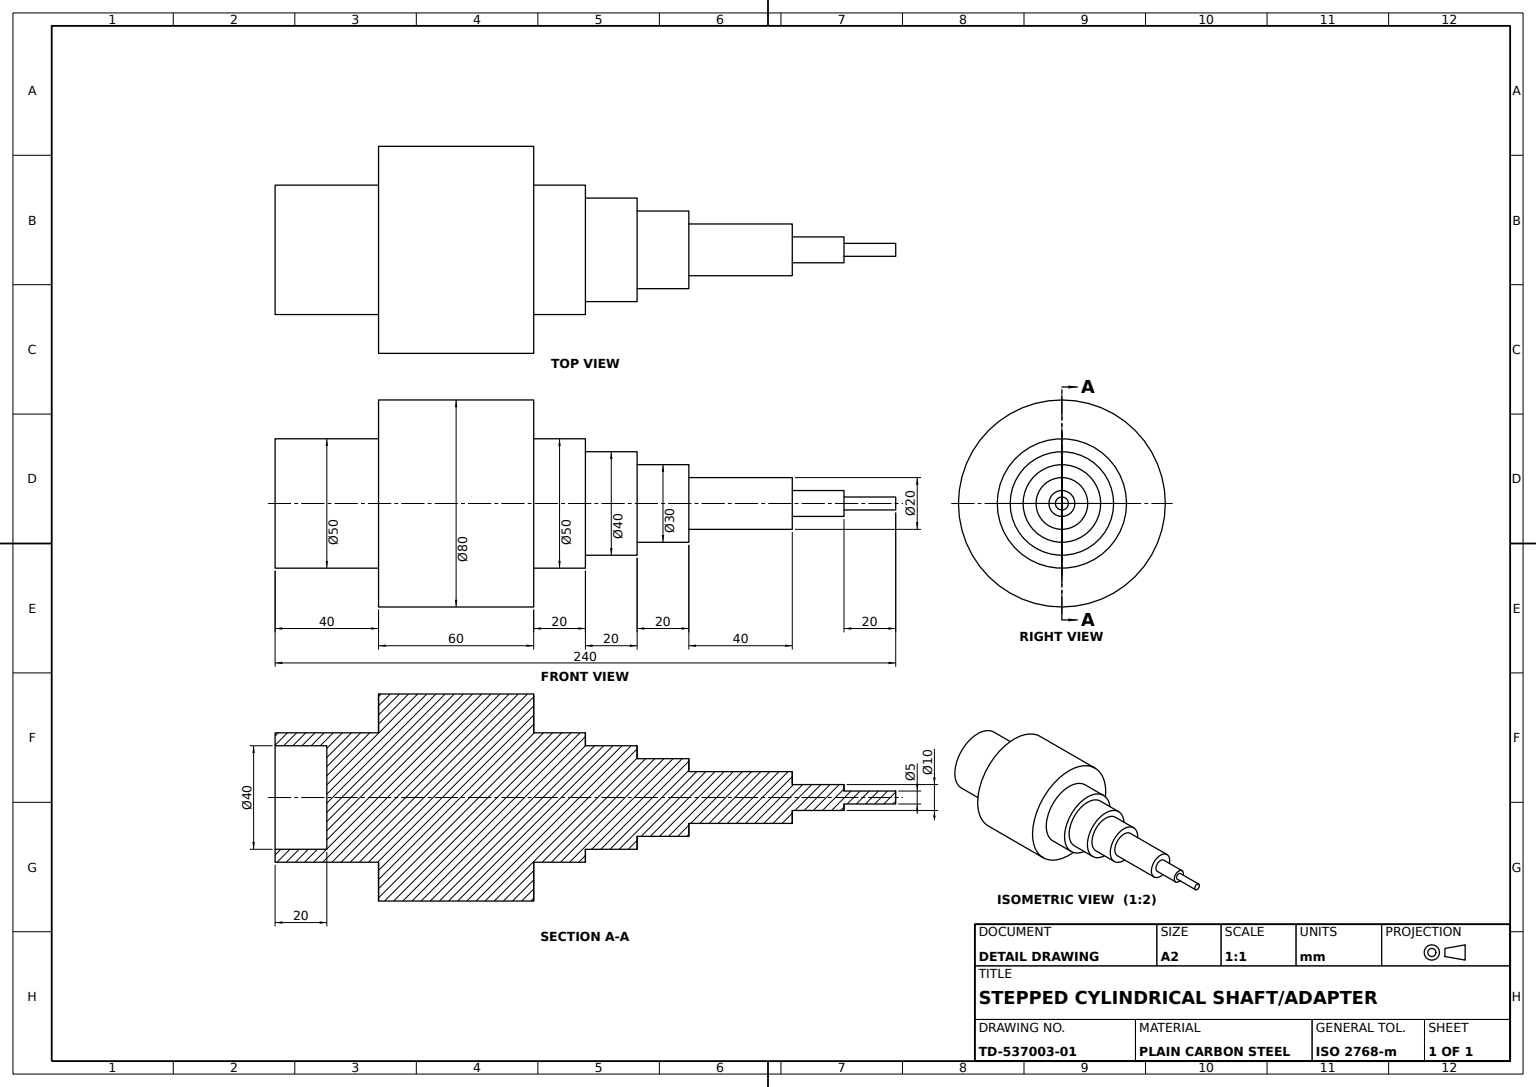
SolidWorks part; units mm, degrees
material "Plain Carbon Steel"
ref_plane "Front Plane" through (0, 0, 0) normal (0, 0, 1) x (1, 0, 0)
ref_plane "Top Plane" through (0, 0, 0) normal (0, 1, 0) x (1, 0, 0)
ref_plane "Right Plane" through (0, 0, 0) normal (1, 0, 0) x (0, 0, -1)
sketch "Collar Profile Ø80" plane through (0, 0, 0) normal (0, 0, 1) x (1, 0, 0)
  line L0 (0, 58.5842) -> (0, -59.3941) construction
  line L1 (-69.9034, 0) -> (92.6205, 0) construction
  circle A0 centre (0, 0) radius 40
  dimension "D1" = 80
extrude "Collar Ø80" add sketch "Collar Profile Ø80" along normal blind 60
sketch "Spigot Sketch Ø50" plane through (0, 0, 60) normal (0, 0, 1) x (1, 0, 0)
  circle A0 centre (0, 0) radius 25
  dimension "D1" = 50
extrude "Spigot Ø50" add sketch "Spigot Sketch Ø50" along normal blind 40
sketch "Spigot Bore Sketch Ø40" plane through (0, 0, 100) normal (0, 0, 1) x (1, 0, 0)
  circle A0 centre (0, 0) radius 20
  dimension "D1" = 40
extrude "Spigot Bore Ø40" cut sketch "Spigot Bore Sketch Ø40" against normal blind 20
sketch "Pin Step 1 Sketch Ø50" plane through (0, 0, 0) normal (0, 0, -1) x (-1, 0, 0)
  circle A0 centre (0, 0) radius 25
  dimension "D1" = 50
extrude "Pin Step 1 Ø50" add sketch "Pin Step 1 Sketch Ø50" along normal blind 20
sketch "Pin Step 2 Sketch Ø40" plane through (0, 0, -20) normal (0, 0, -1) x (-1, 0, 0)
  circle A0 centre (0, 0) radius 20
  dimension "D1" = 40
extrude "Pin Step 2 Ø40" add sketch "Pin Step 2 Sketch Ø40" along normal blind 20
sketch "Pin Step 3 Sketch Ø30" plane through (0, 0, -40) normal (0, 0, -1) x (-1, 0, 0)
  circle A0 centre (0, 0) radius 15
  dimension "D1" = 30
extrude "Pin Step 3 Ø30" add sketch "Pin Step 3 Sketch Ø30" along normal blind 20
sketch "Pin Step 4 Sketch Ø20" plane through (0, 0, -60) normal (0, 0, -1) x (-1, 0, 0)
  circle A0 centre (0, 0) radius 10
  dimension "D1" = 20
extrude "Pin Step 4 Ø20" add sketch "Pin Step 4 Sketch Ø20" along normal blind 20
sketch "Pin Step 5 Sketch Ø20" plane through (0, 0, -80) normal (0, 0, -1) x (-1, 0, 0)
  circle A0 centre (0, 0) radius 10
  dimension "D1" = 20
extrude "Pin Step 5 Ø20" add sketch "Pin Step 5 Sketch Ø20" along normal blind 20
sketch "Pin Step 6 Sketch Ø10" plane through (0, 0, -100) normal (0, 0, -1) x (-1, 0, 0)
  circle A0 centre (0, 0) radius 5
  dimension "D1" = 10
extrude "Pin Step 6 Ø10" add sketch "Pin Step 6 Sketch Ø10" along normal blind 20
sketch "Pin Tip Sketch Ø5" plane through (0, 0, -120) normal (0, 0, -1) x (-1, 0, 0)
  circle A0 centre (0, 0) radius 2.5
  dimension "D1" = 5
extrude "Pin Tip Ø5" add sketch "Pin Tip Sketch Ø5" along normal blind 20
